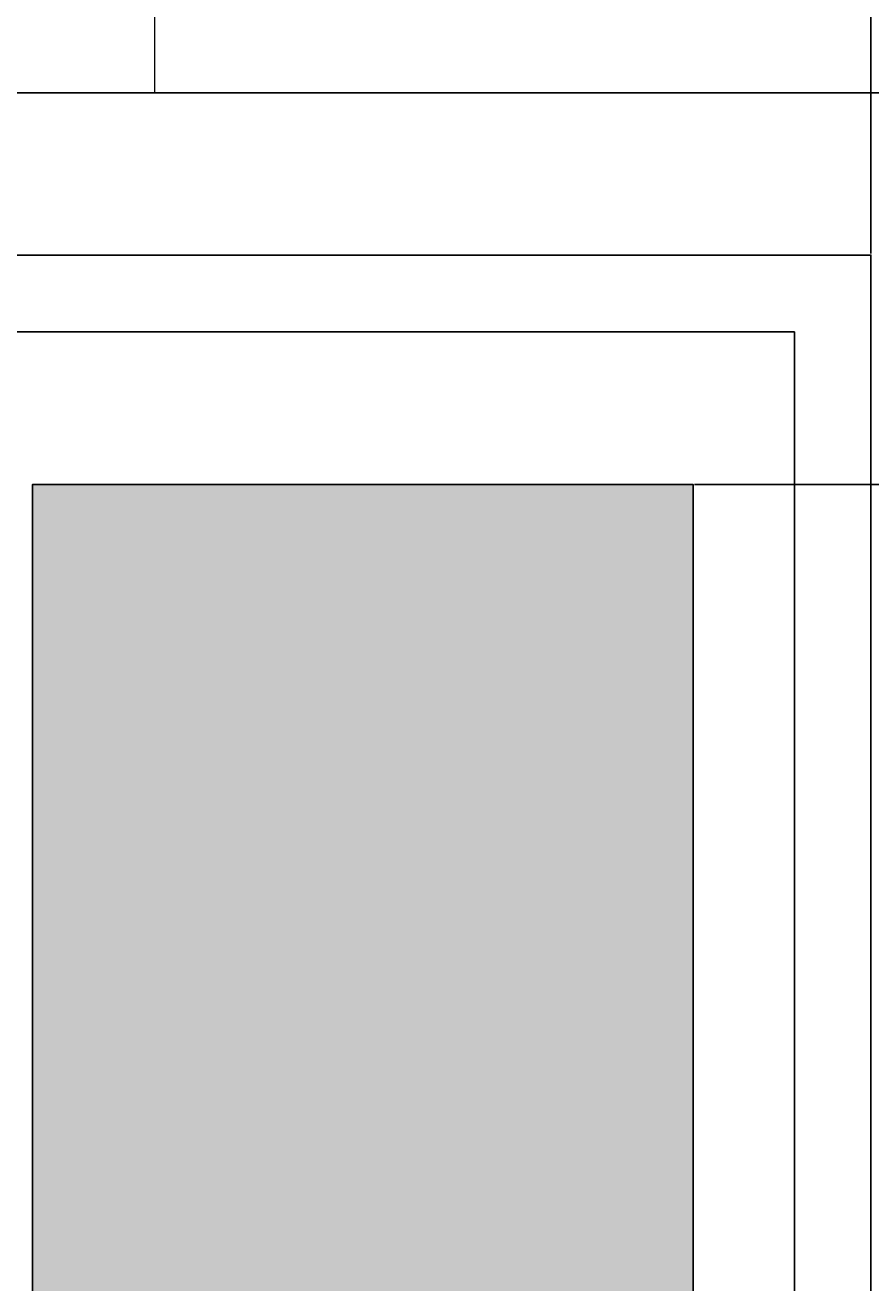
# Model space of a CAD drawing. Units: inches. Extents: x 37 to 824, y -700 to 234.
# Tile 17 of 77: x 315 to 348, y -536 to -487. Entities that reach past the tile are written whole.
import ezdxf

# ---------------------------------------------------------------- set-up
doc = ezdxf.new("R2010")
doc.units = ezdxf.units.IN
doc.header["$MEASUREMENT"] = 0
for name, color, linetype, lineweight in [('A-ANNO-DIMS', 2, 'Continuous', 18), ('A-DOOR', 4, 'Continuous', 25), ('A-ELEV', 3, 'Continuous', 25), ('A-ELEV-PATT', 8, 'Continuous', 13)]:
    doc.layers.add(name, color=color, linetype=linetype, lineweight=lineweight)
doc.styles.get("Standard").update_dxf_attribs({"font": 'arial.ttf'})
doc.dimstyles.get("Standard").update_dxf_attribs({"dimtxt": 0.18, "dimasz": 0.18, "dimexe": 0.18, "dimexo": 0.0625, "dimgap": 0.09, "dimtad": 0, "dimtih": 1, "dimtoh": 1, "dimdec": 1, "dimzin": 0, "dimdsep": 46, "dimlunit": 4, "dimtxsty": 'Standard', "dimcen": 0.09, "dimadec": 0, "dimazin": 0, "dimtfac": 1, "dimtdec": 1, "dimtofl": 0, "dimtmove": 0, "dimatfit": 3, "dimfxl": 1, "dimtolj": 1, "dimtzin": 0, "dimarcsym": 0})

# ---------------------------------------------------------------- blocks, each defined once
blk = doc.blocks.new('*U9')
blk.add_lwpolyline([(3.124, 0.013), (0.124, 0.013), (0.124, 84.013), (40.124, 84.013), (40.124, 0.013), (37.124, 0.013)])
for points in [[(37.124, 80.99), (37.124, 0.013), (3.124, 0.013), (3.124, 80.99)], [(33.124, 6.013), (33.124, 74.99), (7.124, 74.99), (7.124, 6.013)]]:
    blk.add_lwpolyline(points, close=True)
blk = doc.blocks.new('*D31')
at = {"layer": 'A-ANNO-DIMS', "color": 0, "lineweight": -2, "ltscale": 0.5, "transparency": 16777216}
for p, q in [((255.14, -489.627), (449.772, -489.627)), ((449.592, -495.627), (449.592, -510.537)), ((449.592, -531.627), (449.592, -516.717)), ((255.14, -537.627), (449.772, -537.627))]:
    blk.add_line(p, q, dxfattribs=at)
at = {"layer": 'A-ANNO-DIMS', "color": 0, "ltscale": 0.5, "transparency": 16777216}
for points in [[(448.592, -495.627), (450.592, -495.627), (449.592, -489.627)], [(448.592, -531.627), (450.592, -531.627), (449.592, -537.627)]]:
    blk.add_solid(points, dxfattribs=at)
at = {"layer": 'Defpoints', "color": 0, "ltscale": 0.5, "transparency": 16777216}
for p in [(255.077, -489.627), (449.592, -489.627), (255.077, -537.627)]:
    blk.add_point(p, dxfattribs=at)
at = {"layer": 'A-ANNO-DIMS', "color": 0, "ltscale": 0.5, "transparency": 16777216, "insert": (449.592, -513.627), "char_height": 6, "attachment_point": 5}
blk.add_mtext("\\A1;4'", dxfattribs=at)
blk = doc.blocks.new('*D99')
at = {"layer": 'A-ANNO-DIMS', "color": 0, "lineweight": -2, "ltscale": 0.5, "transparency": 16777216}
for p, q in [((308.196, -495.944), (308.196, -378.38)), ((348.196, -495.944), (348.196, -378.38)), ((308.376, -378.56), (327.866, -378.56)), ((348.016, -378.56), (328.525, -378.56))]:
    blk.add_line(p, q, dxfattribs=at)
at = {"layer": 'A-ANNO-DIMS', "color": 0, "ltscale": 0.5, "transparency": 16777216}
for points in [[(308.376, -378.53), (308.376, -378.59), (308.196, -378.56)], [(348.016, -378.53), (348.016, -378.59), (348.196, -378.56)]]:
    blk.add_solid(points, dxfattribs=at)
at = {"layer": 'Defpoints', "color": 0, "ltscale": 0.5, "transparency": 16777216}
for p in [(348.196, -378.56), (308.196, -496.007), (348.196, -496.007)]:
    blk.add_point(p, dxfattribs=at)
at = {"layer": 'A-ANNO-DIMS', "color": 0, "ltscale": 0.5, "transparency": 16777216, "insert": (328.196, -378.56), "char_height": 0.18, "attachment_point": 5}
blk.add_mtext('\\A1;3\'-4"', dxfattribs=at)
blk = doc.blocks.new('*D102')
at = {"layer": 'A-ANNO-DIMS', "color": 0, "lineweight": -2, "ltscale": 0.5, "transparency": 16777216}
for p, q in [((311.196, -499.092), (311.196, -699.594)), ((345.196, -499.092), (345.196, -699.594)), ((311.376, -699.414), (327.795, -699.414)), ((345.016, -699.414), (328.596, -699.414))]:
    blk.add_line(p, q, dxfattribs=at)
at = {"layer": 'A-ANNO-DIMS', "color": 0, "ltscale": 0.5, "transparency": 16777216}
for points in [[(311.376, -699.384), (311.376, -699.444), (311.196, -699.414)], [(345.016, -699.384), (345.016, -699.444), (345.196, -699.414)]]:
    blk.add_solid(points, dxfattribs=at)
at = {"layer": 'Defpoints', "color": 0, "ltscale": 0.5, "transparency": 16777216}
for p in [(311.196, -499.03), (345.196, -499.03), (345.196, -699.414)]:
    blk.add_point(p, dxfattribs=at)
at = {"layer": 'A-ANNO-DIMS', "color": 0, "ltscale": 0.5, "transparency": 16777216, "insert": (328.196, -699.414), "char_height": 0.18, "attachment_point": 5}
blk.add_mtext('\\A1;2\'-10"', dxfattribs=at)
blk = doc.blocks.new('*D103')
at = {"layer": 'A-ANNO-DIMS', "color": 0, "lineweight": -2, "ltscale": 0.5, "transparency": 16777216}
for p, q in [((315.196, -505.092), (315.196, -699.594)), ((341.196, -505.092), (341.196, -699.594)), ((315.376, -699.414), (327.865, -699.414)), ((341.016, -699.414), (328.526, -699.414))]:
    blk.add_line(p, q, dxfattribs=at)
at = {"layer": 'A-ANNO-DIMS', "color": 0, "ltscale": 0.5, "transparency": 16777216}
for points in [[(315.376, -699.384), (315.376, -699.444), (315.196, -699.414)], [(341.016, -699.384), (341.016, -699.444), (341.196, -699.414)]]:
    blk.add_solid(points, dxfattribs=at)
at = {"layer": 'Defpoints', "color": 0, "ltscale": 0.5, "transparency": 16777216}
for p in [(315.196, -505.03), (341.196, -505.03), (341.196, -699.414)]:
    blk.add_point(p, dxfattribs=at)
at = {"layer": 'A-ANNO-DIMS', "color": 0, "ltscale": 0.5, "transparency": 16777216, "insert": (328.196, -699.414), "char_height": 0.18, "attachment_point": 5}
blk.add_mtext('\\A1;2\'-2"', dxfattribs=at)
blk = doc.blocks.new('*D104')
at = {"layer": 'A-ANNO-DIMS', "color": 0, "lineweight": -2, "ltscale": 0.5, "transparency": 16777216}
for p, q in [((341.258, -505.03), (556.923, -505.03)), ((556.743, -505.21), (556.743, -539.336)), ((556.743, -573.827), (556.743, -539.7)), ((341.258, -574.007), (556.923, -574.007))]:
    blk.add_line(p, q, dxfattribs=at)
at = {"layer": 'A-ANNO-DIMS', "color": 0, "ltscale": 0.5, "transparency": 16777216}
for points in [[(556.713, -505.21), (556.773, -505.21), (556.743, -505.03)], [(556.713, -573.827), (556.773, -573.827), (556.743, -574.007)]]:
    blk.add_solid(points, dxfattribs=at)
at = {"layer": 'Defpoints', "color": 0, "ltscale": 0.5, "transparency": 16777216}
for p in [(341.196, -505.03), (341.196, -574.007), (556.743, -574.007)]:
    blk.add_point(p, dxfattribs=at)
at = {"layer": 'A-ANNO-DIMS', "color": 0, "ltscale": 0.5, "transparency": 16777216, "insert": (556.743, -539.518), "char_height": 0.18, "attachment_point": 5}
blk.add_mtext('\\A1;5\'-9"', dxfattribs=at)

msp = doc.modelspace()

# ---------------------------------------------------------------- hatches: boundary and pattern name
at = {"layer": 'A-ELEV-PATT', "ltscale": 0.5}
h = msp.add_hatch(color=256, dxfattribs=at)
h.dxf.hatch_style = 1
h.paths.add_polyline_path([(161.077, -459.627), (161.077, -465.627), (428.077, -465.627), (428.077, -459.627)])
h.paths.add_polyline_path([(229.025, -498.214), (214.525, -498.214), (214.525, -529.214), (229.025, -529.214)])
h.paths.add_polyline_path([(245.525, -498.214), (230.025, -498.214), (230.025, -529.214), (245.525, -529.214)])
h.paths.add_polyline_path([(315.196, -574.007), (341.196, -574.007), (341.196, -505.03), (315.196, -505.03)])
h = msp.add_hatch(dxfattribs=at)
h.set_pattern_fill('AR-BRSTD', color=256, scale=4)
h.paths.add_polyline_path([(299.077, -489.627), (358.132, -489.627), (358.132, -585.627), (428.077, -585.627), (428.077, -465.627), (161.077, -465.627), (161.077, -585.627), (299.077, -585.627)])
h.paths.add_polyline_path([(205.077, -537.627), (205.077, -489.627), (255.077, -489.627), (255.077, -537.627)], flags=16)

# ---------------------------------------------------------------- linework, layer by layer
at = {"layer": 'A-ELEV', "ltscale": 0.5}
msp.add_lwpolyline([(299.077, -489.627), (358.132, -489.627), (358.132, -585.627), (299.077, -585.627)], close=True, dxfattribs=at)

# ---------------------------------------------------------------- block references
at = {"layer": 'A-DOOR'}
msp.add_blockref('*U9', (308.072, -580.019), dxfattribs=at)

# ---------------------------------------------------------------- dimensions: what is measured, and where the dimension line sits
at = {"layer": 'A-ANNO-DIMS', "ltscale": 0.5}
for base, p1, p2, picture, middle in [((348.196, -378.56), (308.196, -496.007), (348.196, -496.007), '*D99', (328.196, -378.56)), ((345.196, -699.414), (311.196, -499.03), (345.196, -499.03), '*D102', (328.196, -699.414)), ((341.196, -699.414), (315.196, -505.03), (341.196, -505.03), '*D103', (328.196, -699.414))]:
    dim = msp.add_linear_dim(base=base, p1=p1, p2=p2, dimstyle='Standard', override={"dimdec": 1, "dimlfac": 1, "dimrnd": 0, "dimzin": 1, "dimdsep": 46, "dimlunit": 4, "dimfrac": 2}, dxfattribs=at)
    dim.commit()
    dim.dimension.update_dxf_attribs({"geometry": picture, "text_midpoint": middle})
for base, p1, p2, override, picture, middle in [((449.592, -489.627), (255.077, -537.627), (255.077, -489.627), {"dimtxt": 6, "dimasz": 6, "dimclrd": 0, "dimclre": 0, "dimclrt": 0}, '*D31', (449.592, -513.627)), ((556.743, -574.007), (341.196, -505.03), (341.196, -574.007), {"dimdec": 1, "dimlfac": 1, "dimrnd": 0, "dimzin": 1, "dimdsep": 46, "dimlunit": 4, "dimfrac": 2}, '*D104', (556.743, -539.518))]:
    dim = msp.add_linear_dim(base=base, p1=p1, p2=p2, angle=90, dimstyle='Standard', override=override, dxfattribs=at)
    dim.commit()
    dim.dimension.update_dxf_attribs({"geometry": picture, "text_midpoint": middle})

doc.saveas('drawing.dxf')
